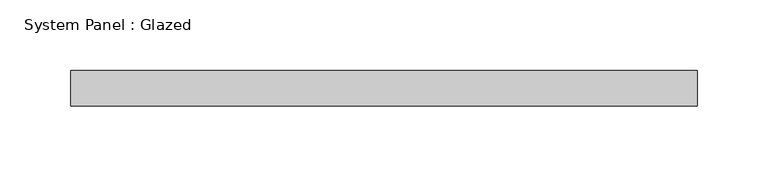
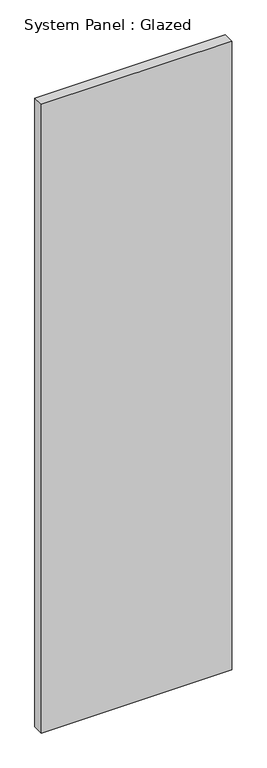
"""IFC4 building model written with IfcOpenShell, lengths in millimetres: plate geometry, System Panel : Glazed."""

from ifc_helpers import new_model, si_unit, origin, origin_with_axes, place, context, project, spatial, polyline, outline, extrude, source, transform, mapped, element, save


def system_panel_glazed_1157894c(model_context):
    return source(origin(), model_context, "Body", "SweptSolid", [
        extrude(outline(polyline([(222.25, 19.05), (-222.25, 19.05), (-222.25, 44.45), (222.25, 44.45), (222.25, 19.05)])), origin_with_axes(), (0.0, 0.0, 1.0), 1550.4900448),
    ])


if __name__ == "__main__":
    model = new_model("IFC4")
    model_context = context("Model", 3, world=origin())
    ifc_project = project(units=[si_unit("LENGTHUNIT", "METRE", prefix="MILLI")], contexts=[model_context])
    site = spatial("IfcSite", under=ifc_project)
    building = spatial("IfcBuilding", under=site)
    placement = place(None, origin())
    system_panel_glazed_shape = system_panel_glazed_1157894c(model_context)
    element("IfcPlate", 1, ObjectType="System Panel : Glazed", at=placement, inside=building, context=model_context, shape_type="MappedRepresentation", body=[
        mapped(system_panel_glazed_shape, transform((0.0, 0.0, 0.0), x_axis=(1.0, 0.0, 0.0), y_axis=(0.0, 1.0, 0.0), z_axis=(0.0, 0.0, 1.0))),
    ])
    save(model, "model.ifc")

# Revit data of these elements
# Type "System Panel : Glazed"
#   Construction Type Id = "GSP4R"
#   Analytic Construction = "1/8 in Pilkington single glazing"
#   Visual Light Transmittance = 0.9
#   Solar Heat Gain Coefficient = 0.86
#   Heat Transfer Coefficient (U) = 1.18115 BTU/(h·ft²·°F)
#   Define Thermal Properties by = 1
# Element 1 (IfcPlate, "System Panel : Glazed")
#   Materials on its faces: "Glass"
# Materials
#   "Glass": class "Glass", colour RGB 0 128 192, transparency 0.75, Description = "Soda Lime Glass", Cost = 0
